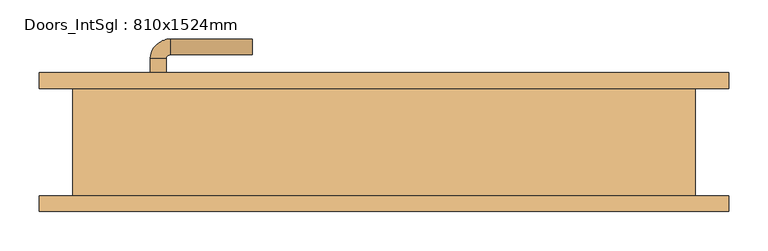
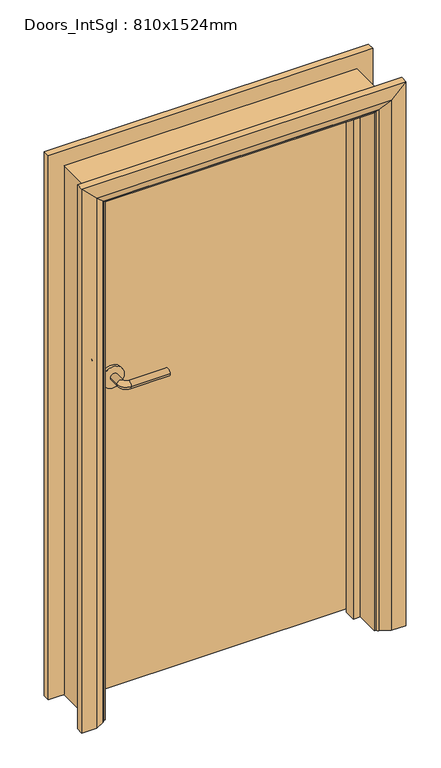
"""IFC4 building model written with IfcOpenShell, lengths in millimetres: door geometry, Doors_IntSgl : 810x1524mm."""

from ifc_helpers import new_model, si_unit, point, frame, frame_2d, origin, place, context, project, spatial, polyline, circle_curve, ellipse_curve, trimmed, segment, composite_curve, outline, extrude, faceted_brep, source, transform, mapped, element, save
from ifc_brep_helpers import plane_surface, cylinder_surface, revolved_surface, advanced_brep


def doors_intsgl_810x1524mm_3577b09a(model_context):
    return source(origin(), model_context, "Body", "SolidModel", [
        advanced_brep(
        [(-298.0, 22.58, 900.0), (-278.0, 22.58, 900.0), (-278.0, -7.42, 900.0), (-298.0, -7.42, 900.0), (-273.0, -12.42, 900.0), (-273.0, -32.42, 900.0), (-168.0, -32.42, 900.0), (-168.0, -12.42, 900.0)],
        [
            (0, 1, circle_curve(frame((-288.0, 22.58, 900.0), z_axis=(0.0, 1.0, 0.0), x_axis=(1.0, 0.0, 0.0)), 10.0)),
            (1, 0, circle_curve(frame((-288.0, 22.58, 900.0), z_axis=(0.0, 1.0, 0.0), x_axis=(1.0, 0.0, 0.0)), 10.0)),
            (1, 2),
            (2, 3, circle_curve(frame((-288.0, -7.42, 900.0), z_axis=(0.0, 1.0, 0.0), x_axis=(1.0, 0.0, 0.0)), 10.0)),
            (3, 0),
            (3, 2, circle_curve(frame((-288.0, -7.42, 900.0), z_axis=(0.0, 1.0, 0.0), x_axis=(1.0, 0.0, 0.0)), 10.0)),
            (4, 5, circle_curve(frame((-273.0, -22.42, 900.0), z_axis=(-1.0, 0.0, 0.0), x_axis=(0.0, 1.0, 0.0)), 10.0)),
            (5, 3, circle_curve(frame((-273.0, -7.42, 900.0), z_axis=(0.0, 0.0, -1.0), x_axis=(-1.0, 0.0, 0.0)), 25.0)),
            (2, 4, circle_curve(frame((-273.0, -7.42, 900.0), z_axis=(0.0, 0.0, 1.0), x_axis=(-1.0, 0.0, 0.0)), 5.0)),
            (5, 4, circle_curve(frame((-273.0, -22.42, 900.0), z_axis=(-1.0, 0.0, 0.0), x_axis=(0.0, 1.0, 0.0)), 10.0)),
            (6, 7, circle_curve(frame((-168.0, -22.42, 900.0), z_axis=(1.0, 0.0, 0.0), x_axis=(0.0, 1.0, 0.0)), 10.0)),
            (7, 6, circle_curve(frame((-168.0, -22.42, 900.0), z_axis=(1.0, 0.0, 0.0), x_axis=(0.0, 1.0, 0.0)), 10.0)),
            (4, 7),
            (6, 5),
        ],
        [
            plane_surface(frame((-288.0, 22.58, 900.0), z_axis=(0.0, 1.0, 0.0), x_axis=(0.0, 0.0, 1.0))),
            cylinder_surface(frame((-288.0, 22.58, 900.0), z_axis=(0.0, 1.0, 0.0), x_axis=(1.0, 0.0, 0.0)), 10.0),
            revolved_surface(trimmed(ellipse_curve(frame((-288.0, -7.42, 900.0), z_axis=(0.0, -1.0, 0.0), x_axis=(1.0, 0.0, 0.0)), 10.0, 10.0), [point((-298.0, -7.42, 900.0))], [point((-278.0, -7.42, 900.0))], True, "CARTESIAN"), (-273.0, -7.42, 900.0), (0.0, 0.0, -1.0)),
            revolved_surface(trimmed(ellipse_curve(frame((-288.0, -7.42, 900.0), z_axis=(0.0, -1.0, 0.0), x_axis=(1.0, 0.0, 0.0)), 10.0, 10.0), [point((-278.0, -7.42, 900.0))], [point((-298.0, -7.42, 900.0))], True, "CARTESIAN"), (-273.0, -7.42, 900.0), (0.0, 0.0, -1.0)),
            plane_surface(frame((-168.0, -22.42, 900.0), z_axis=(1.0, 0.0, 0.0), x_axis=(0.0, 0.0, 1.0))),
            cylinder_surface(frame((-273.0, -22.42, 900.0), z_axis=(-1.0, 0.0, 0.0), x_axis=(0.0, 1.0, 0.0)), 10.0),
        ],
        [
            (0, [[1, 2]]),
            (1, [[3, 4, 5, -2]]),
            (1, [[-5, 6, -3, -1]]),
            (2, [[7, 8, -4, 9]]),
            (3, [[10, -9, -6, -8]]),
            (4, [[11, 12]]),
            (5, [[13, -11, 14, -7]]),
            (5, [[-14, -12, -13, -10]]),
        ],
    ),
        extrude(outline(composite_curve([segment(trimmed(circle_curve(frame_2d((900.0, -290.5)), 30.0), [point((900.0, -320.5))], [point((900.0, -260.5))], False, "CARTESIAN"), True, "CONTINUOUS"), segment(trimmed(circle_curve(frame_2d((900.0, -290.5)), 30.0), [point((900.0, -260.5))], [point((900.0, -320.5))], False, "CARTESIAN"), True, "CONTINUOUS")], self_intersect=False)), frame((0.0, 22.58, 0.0), z_axis=(0.0, 1.0, 0.0), x_axis=(0.0, 0.0, 1.0)), (0.0, 0.0, 1.0), 8.0),
        advanced_brep(
        [(-298.0, 76.58, 900.0), (-278.0, 76.58, 900.0), (-298.0, 106.58, 900.0), (-278.0, 106.58, 900.0), (-273.0, 111.58, 900.0), (-273.0, 131.58, 900.0), (-168.0, 131.58, 900.0), (-168.0, 111.58, 900.0)],
        [
            (0, 1, circle_curve(frame((-288.0, 76.58, 900.0), z_axis=(0.0, -1.0, 0.0), x_axis=(1.0, 0.0, 0.0)), 10.0)),
            (1, 0, circle_curve(frame((-288.0, 76.58, 900.0), z_axis=(0.0, -1.0, 0.0), x_axis=(1.0, 0.0, 0.0)), 10.0)),
            (0, 2),
            (2, 3, circle_curve(frame((-288.0, 106.58, 900.0), z_axis=(0.0, -1.0, 0.0), x_axis=(1.0, 0.0, 0.0)), 10.0)),
            (3, 1),
            (3, 2, circle_curve(frame((-288.0, 106.58, 900.0), z_axis=(0.0, -1.0, 0.0), x_axis=(1.0, 0.0, 0.0)), 10.0)),
            (4, 3, circle_curve(frame((-273.0, 106.58, 900.0), z_axis=(0.0, 0.0, 1.0), x_axis=(-1.0, 0.0, 0.0)), 5.0)),
            (2, 5, circle_curve(frame((-273.0, 106.58, 900.0), z_axis=(0.0, 0.0, -1.0), x_axis=(-1.0, 0.0, 0.0)), 25.0)),
            (5, 4, circle_curve(frame((-273.0, 121.58, 900.0), z_axis=(-1.0, 0.0, 0.0), x_axis=(0.0, -1.0, 0.0)), 10.0)),
            (4, 5, circle_curve(frame((-273.0, 121.58, 900.0), z_axis=(-1.0, 0.0, 0.0), x_axis=(0.0, -1.0, 0.0)), 10.0)),
            (6, 7, circle_curve(frame((-168.0, 121.58, 900.0), z_axis=(1.0, 0.0, 0.0), x_axis=(0.0, -1.0, 0.0)), 10.0)),
            (7, 6, circle_curve(frame((-168.0, 121.58, 900.0), z_axis=(1.0, 0.0, 0.0), x_axis=(0.0, -1.0, 0.0)), 10.0)),
            (5, 6),
            (7, 4),
        ],
        [
            plane_surface(frame((-288.0, 76.58, 900.0), z_axis=(0.0, -1.0, 0.0), x_axis=(0.0, 0.0, 1.0))),
            cylinder_surface(frame((-288.0, 76.58, 900.0), z_axis=(0.0, -1.0, 0.0), x_axis=(1.0, 0.0, 0.0)), 10.0),
            revolved_surface(trimmed(ellipse_curve(frame((-288.0, 106.58, 900.0), z_axis=(0.0, -1.0, 0.0), x_axis=(1.0, 0.0, 0.0)), 10.0, 10.0), [point((-298.0, 106.58, 900.0))], [point((-278.0, 106.58, 900.0))], True, "CARTESIAN"), (-273.0, 106.58, 900.0), (0.0, 0.0, -1.0)),
            revolved_surface(trimmed(ellipse_curve(frame((-288.0, 106.58, 900.0), z_axis=(0.0, -1.0, 0.0), x_axis=(1.0, 0.0, 0.0)), 10.0, 10.0), [point((-278.0, 106.58, 900.0))], [point((-298.0, 106.58, 900.0))], True, "CARTESIAN"), (-273.0, 106.58, 900.0), (0.0, 0.0, -1.0)),
            plane_surface(frame((-168.0, 121.58, 900.0), z_axis=(1.0, 0.0, 0.0), x_axis=(0.0, 0.0, 1.0))),
            cylinder_surface(frame((-273.0, 121.58, 900.0), z_axis=(-1.0, 0.0, 0.0), x_axis=(0.0, -1.0, 0.0)), 10.0),
        ],
        [
            (0, [[1, 2]]),
            (1, [[-1, 3, 4, 5]]),
            (1, [[-2, -5, 6, -3]]),
            (2, [[7, -4, 8, 9]]),
            (3, [[-8, -6, -7, 10]]),
            (4, [[11, 12]]),
            (5, [[-9, 13, -12, 14]]),
            (5, [[-10, -14, -11, -13]]),
        ],
    ),
        extrude(outline(composite_curve([segment(trimmed(circle_curve(frame_2d((900.0, -290.5)), 30.0), [point((900.0, -320.5))], [point((900.0, -260.5))], False, "CARTESIAN"), True, "CONTINUOUS"), segment(trimmed(circle_curve(frame_2d((900.0, -290.5)), 30.0), [point((900.0, -260.5))], [point((900.0, -320.5))], False, "CARTESIAN"), True, "CONTINUOUS")], self_intersect=False)), frame((0.0, 68.58, 0.0), z_axis=(0.0, 1.0, 0.0), x_axis=(0.0, 0.0, 1.0)), (0.0, 0.0, 1.0), 8.0),
        extrude(outline(polyline([(363.0, 30.58), (-363.0, 30.58), (-363.0, 68.58), (363.0, 68.58), (363.0, 30.58)])), frame((0.0, 0.0, 8.0), z_axis=(0.0, 0.0, 1.0), x_axis=(1.0, 0.0, 0.0)), (0.0, 0.0, 1.0), 1474.0),
        advanced_brep(
        [(440.0, 88.58, 0.0), (440.0, 68.58, 0.0), (370.0, 68.58, 0.0), (374.0, 74.58, 0.0), (400.0, 88.58, 0.0), (440.0, 88.58, 1559.0), (440.0, 68.58, 1559.0), (-440.0, 68.58, 1559.0), (-440.0, 68.58, 0.0), (-370.0, 68.58, 0.0), (-370.0, 68.58, 1489.0), (370.0, 68.58, 1489.0), (374.0, 74.58, 1493.0), (400.0, 88.58, 1519.0), (-400.0, 88.58, 1519.0), (-400.0, 88.58, 0.0), (-440.0, 88.58, 0.0), (-440.0, 88.58, 1559.0), (-374.0, 74.58, 1493.0), (-374.0, 74.58, 0.0)],
        [
            (0, 1),
            (1, 2),
            (2, 3, circle_curve(frame((378.0, 67.58, 0.0), z_axis=(0.0, 0.0, -1.0), x_axis=(1.0, 0.0, 0.0)), 8.0622577)),
            (3, 4),
            (4, 0),
            (0, 5),
            (5, 6),
            (6, 1),
            (6, 7),
            (7, 8),
            (8, 9),
            (9, 10),
            (10, 11),
            (11, 2),
            (11, 12, ellipse_curve(frame((378.0, 67.58, 1497.0), z_axis=(0.7071067811865475, 0.0, -0.7071067811865475), x_axis=(-0.7071067811865474, 0.0, -0.7071067811865476)), 11.4017543, 8.0622577)),
            (12, 3),
            (12, 13),
            (13, 4),
            (13, 14),
            (14, 15),
            (15, 16),
            (16, 17),
            (17, 5),
            (17, 7),
            (10, 18, ellipse_curve(frame((-378.0, 67.58, 1497.0), z_axis=(0.7071067811865475, 0.0, 0.7071067811865475), x_axis=(0.7071067811865476, 0.0, -0.7071067811865474)), 11.4017543, 8.0622577)),
            (18, 12),
            (18, 14),
            (15, 19),
            (19, 9, circle_curve(frame((-378.0, 67.58, 0.0), z_axis=(0.0, 0.0, -1.0), x_axis=(-1.0, 0.0, 0.0)), 8.0622577)),
            (8, 16),
            (19, 18),
        ],
        [
            plane_surface(frame((370.0, 68.58, 0.0), z_axis=(0.0, 0.0, -1.0), x_axis=(0.0, -1.0, 0.0))),
            plane_surface(frame((440.0, 88.58, 0.0), z_axis=(1.0, 0.0, 0.0), x_axis=(0.0, 0.0, 1.0))),
            plane_surface(frame((440.0, 68.58, 0.0), z_axis=(0.0, -1.0, 0.0), x_axis=(0.0, 0.0, 1.0))),
            cylinder_surface(frame((378.0, 67.58, 0.0), z_axis=(0.0, 0.0, -1.0), x_axis=(1.0, 0.0, 0.0)), 8.0622577),
            plane_surface(frame((374.0, 74.58, 0.0), z_axis=(-0.4740998230350126, 0.880471099922178, 0.0), x_axis=(0.0, 0.0, 1.0))),
            plane_surface(frame((400.0, 88.58, 0.0), z_axis=(0.0, 1.0, 0.0), x_axis=(0.0, 0.0, 1.0))),
            plane_surface(frame((440.0, 88.58, 1559.0), z_axis=(0.0, 0.0, 1.0), x_axis=(-1.0, 0.0, 0.0))),
            cylinder_surface(frame((370.0, 67.58, 1497.0), z_axis=(1.0, 0.0, 0.0), x_axis=(0.0, 0.0, 1.0)), 8.0622577),
            plane_surface(frame((374.0, 74.58, 1493.0), z_axis=(0.0, 0.8804710999221764, -0.4740998230350154), x_axis=(-1.0, 0.0, 0.0))),
            plane_surface(frame((-370.0, 68.58, 0.0), z_axis=(0.0, 0.0, -1.0), x_axis=(0.0, -1.0, 0.0))),
            plane_surface(frame((-440.0, 88.58, 1559.0), z_axis=(-1.0, 0.0, 0.0), x_axis=(0.0, 0.0, -1.0))),
            cylinder_surface(frame((-378.0, 67.58, 1489.0), z_axis=(0.0, 0.0, 1.0), x_axis=(-1.0, 0.0, 0.0)), 8.0622577),
            plane_surface(frame((-374.0, 74.58, 1493.0), z_axis=(0.47409982303501824, 0.8804710999221749, 0.0), x_axis=(0.0, 0.0, -1.0))),
        ],
        [
            (0, [[1, 2, 3, 4, 5]]),
            (1, [[-1, 6, 7, 8]]),
            (2, [[-2, -8, 9, 10, 11, 12, 13, 14]]),
            (3, [[-3, -14, 15, 16]]),
            (4, [[-4, -16, 17, 18]]),
            (5, [[-5, -18, 19, 20, 21, 22, 23, -6]]),
            (6, [[-7, -23, 24, -9]]),
            (7, [[-15, -13, 25, 26]]),
            (8, [[-17, -26, 27, -19]]),
            (9, [[-21, 28, 29, -11, 30]]),
            (10, [[-24, -22, -30, -10]]),
            (11, [[-25, -12, -29, 31]]),
            (12, [[-27, -31, -28, -20]]),
        ],
    ),
        advanced_brep(
        [(-440.0, -88.58, 0.0), (-440.0, -68.58, 0.0), (-370.0, -68.58, 0.0), (-374.0, -74.58, 0.0), (-400.0, -88.58, 0.0), (-440.0, -88.58, 1559.0), (-440.0, -68.58, 1559.0), (-370.0, -68.58, 1489.0), (-374.0, -74.58, 1493.0), (-400.0, -88.58, 1519.0), (440.0, -88.58, 1559.0), (440.0, -68.58, 1559.0), (370.0, -68.58, 1489.0), (374.0, -74.58, 1493.0), (400.0, -88.58, 1519.0), (440.0, -88.58, 0.0), (400.0, -88.58, 0.0), (374.0, -74.58, 0.0), (370.0, -68.58, 0.0), (440.0, -68.58, 0.0)],
        [
            (0, 1),
            (1, 2),
            (2, 3, circle_curve(frame((-378.0, -67.58, 0.0), z_axis=(0.0, 0.0, -1.0), x_axis=(-1.0, 0.0, 0.0)), 8.0622577)),
            (3, 4),
            (4, 0),
            (0, 5),
            (5, 6),
            (6, 1),
            (6, 7),
            (7, 2),
            (7, 8, ellipse_curve(frame((-378.0, -67.58, 1497.0), z_axis=(-0.7071067811865475, 0.0, -0.7071067811865475), x_axis=(0.7071067811865474, 0.0, -0.7071067811865476)), 11.4017543, 8.0622577)),
            (8, 3),
            (8, 9),
            (9, 4),
            (9, 5),
            (5, 10),
            (10, 11),
            (11, 6),
            (11, 12),
            (12, 7),
            (12, 13, ellipse_curve(frame((378.0, -67.58, 1497.0), z_axis=(-0.7071067811865475, 0.0, 0.7071067811865475), x_axis=(-0.7071067811865476, 0.0, -0.7071067811865474)), 11.4017543, 8.0622577)),
            (13, 8),
            (13, 14),
            (14, 9),
            (14, 10),
            (15, 16),
            (16, 17),
            (17, 18, circle_curve(frame((378.0, -67.58, 0.0), z_axis=(0.0, 0.0, -1.0), x_axis=(1.0, 0.0, 0.0)), 8.0622577)),
            (18, 19),
            (19, 15),
            (10, 15),
            (19, 11),
            (18, 12),
            (17, 13),
            (16, 14),
        ],
        [
            plane_surface(frame((-370.0, -141.3810989, 0.0), z_axis=(0.0, 0.0, -1.0), x_axis=(1.0, 0.0, 0.0))),
            plane_surface(frame((-440.0, -88.58, 0.0), z_axis=(-1.0, 0.0, 0.0), x_axis=(0.0, 0.0, 1.0))),
            plane_surface(frame((-440.0, -68.58, 0.0), z_axis=(0.0, 1.0, 0.0), x_axis=(0.0, 0.0, 1.0))),
            cylinder_surface(frame((-378.0, -67.58, 0.0), z_axis=(0.0, 0.0, -1.0), x_axis=(-1.0, 0.0, 0.0)), 8.0622577),
            plane_surface(frame((-374.0, -74.58, 0.0), z_axis=(0.4740998230350183, -0.8804710999221749, 0.0), x_axis=(0.0, 0.0, 1.0))),
            plane_surface(frame((-400.0, -88.58, 0.0), z_axis=(0.0, -1.0, 0.0), x_axis=(0.0, 0.0, 1.0))),
            plane_surface(frame((-440.0, -88.58, 1559.0), z_axis=(0.0, 0.0, 1.0), x_axis=(1.0, 0.0, 0.0))),
            plane_surface(frame((-440.0, -68.58, 1559.0), z_axis=(0.0, 1.0, 0.0), x_axis=(1.0, 0.0, 0.0))),
            cylinder_surface(frame((-370.0, -67.58, 1497.0), z_axis=(-1.0, 0.0, 0.0), x_axis=(0.0, 0.0, 1.0)), 8.0622577),
            plane_surface(frame((-374.0, -74.58, 1493.0), z_axis=(0.0, -0.8804710999221749, -0.4740998230350183), x_axis=(1.0, 0.0, 0.0))),
            plane_surface(frame((-400.0, -88.58, 1519.0), z_axis=(0.0, -1.0, 0.0), x_axis=(1.0, 0.0, 0.0))),
            plane_surface(frame((370.0, -141.3810989, 0.0), z_axis=(0.0, 0.0, -1.0), x_axis=(-1.0, 0.0, 0.0))),
            plane_surface(frame((440.0, -88.58, 1559.0), z_axis=(1.0, 0.0, 0.0), x_axis=(0.0, 0.0, -1.0))),
            plane_surface(frame((440.0, -68.58, 1559.0), z_axis=(0.0, 1.0, 0.0), x_axis=(0.0, 0.0, -1.0))),
            cylinder_surface(frame((378.0, -67.58, 1489.0), z_axis=(0.0, 0.0, 1.0), x_axis=(1.0, 0.0, 0.0)), 8.0622577),
            plane_surface(frame((374.0, -74.58, 1493.0), z_axis=(-0.4740998230350183, -0.8804710999221749, 0.0), x_axis=(0.0, 0.0, -1.0))),
            plane_surface(frame((400.0, -88.58, 1519.0), z_axis=(0.0, -1.0, 0.0), x_axis=(0.0, 0.0, -1.0))),
        ],
        [
            (0, [[1, 2, 3, 4, 5]]),
            (1, [[-1, 6, 7, 8]]),
            (2, [[-2, -8, 9, 10]]),
            (3, [[-3, -10, 11, 12]]),
            (4, [[-4, -12, 13, 14]]),
            (5, [[-5, -14, 15, -6]]),
            (6, [[-7, 16, 17, 18]]),
            (7, [[-9, -18, 19, 20]]),
            (8, [[-11, -20, 21, 22]]),
            (9, [[-13, -22, 23, 24]]),
            (10, [[-15, -24, 25, -16]]),
            (11, [[26, 27, 28, 29, 30]]),
            (12, [[-17, 31, -30, 32]]),
            (13, [[-19, -32, -29, 33]]),
            (14, [[-21, -33, -28, 34]]),
            (15, [[-23, -34, -27, 35]]),
            (16, [[-25, -35, -26, -31]]),
        ],
    ),
        faceted_brep([(-365.0, 68.58, 0.0), (-365.0, -68.58, 0.0), (-397.0, -68.58, 0.0), (-397.0, 68.58, 0.0), (-365.0, 68.58, 1484.0), (-365.0, -68.58, 1484.0), (-397.0, -68.58, 1516.0), (-397.0, 68.58, 1516.0), (365.0, 68.58, 1484.0), (365.0, -68.58, 1484.0), (397.0, -68.58, 1516.0), (397.0, 68.58, 1516.0), (365.0, 68.58, 0.0), (397.0, 68.58, 0.0), (397.0, -68.58, 0.0), (365.0, -68.58, 0.0)], [[[0, 1, 2, 3]], [[1, 0, 4, 5]], [[2, 1, 5, 6]], [[3, 2, 6, 7]], [[0, 3, 7, 4]], [[5, 4, 8, 9]], [[6, 5, 9, 10]], [[7, 6, 10, 11]], [[4, 7, 11, 8]], [[12, 13, 14, 15]], [[9, 8, 12, 15]], [[10, 9, 15, 14]], [[11, 10, 14, 13]], [[8, 11, 13, 12]]]),
        extrude(outline(polyline([(0.0, -365.0), (0.0, -346.0), (1465.0, -346.0), (1465.0, 346.0), (0.0, 346.0), (0.0, 365.0), (1484.0, 365.0), (1484.0, -365.0), (0.0, -365.0)])), frame((0.0, -3.42, 0.0), z_axis=(0.0, 1.0, 0.0), x_axis=(0.0, 0.0, 1.0)), (0.0, 0.0, 1.0), 32.0),
    ])


if __name__ == "__main__":
    model = new_model("IFC4")
    model_context = context("Model", 3, world=origin())
    ifc_project = project(units=[si_unit("LENGTHUNIT", "METRE", prefix="MILLI")], contexts=[model_context])
    site = spatial("IfcSite", under=ifc_project)
    building = spatial("IfcBuilding", under=site)
    placement = place(None, origin())
    doors_intsgl_810x1524mm_shape = doors_intsgl_810x1524mm_3577b09a(model_context)
    element("IfcDoor", 1, ObjectType="Doors_IntSgl : 810x1524mm", at=placement, inside=building, context=model_context, shape_type="MappedRepresentation", body=[
        mapped(doors_intsgl_810x1524mm_shape, transform((0.0, 0.0, 0.0), x_axis=(1.0, 0.0, 0.0), y_axis=(0.0, 1.0, 0.0), z_axis=(0.0, 0.0, 1.0))),
    ])
    save(model, "model.ifc")

# Revit data of these elements
# Type "Doors_IntSgl : 810x1524mm"
#   Construction Type Id = "MDOOR"
#   Type Mark = "42"
#   Type Comments = "Internal Single"
#   Operation = "SingleSwingRight"
#   Manufacturer = "Revit"
#   Keynote = "L20"
#   Description = "Internal Single Door"
#   Analytic Construction = "Metal"
#   UnderCut = 8 mm
#   Tolerance = 2 mm
#   Thickness = 38 mm
#   Thermal Resistance (R) = 0.270117 (m²·K)/W
#   Structural Tolerance = 8 mm
#   StopDepth = 32 mm
#   Stop Thickness = 19 mm
#   Rough Width = 810 mm
#   Rough Height = 1524 mm
#   Height to Top Lock Rail = 1000 mm
#   Heat Transfer Coefficient (U) = 3.7021 W/(m²·K)
#   Handle Z Distance = 900 mm
#   Handle X Distance = 75 mm
#   Frame Thickness = 32 mm
#   Door Panel Width = 726 mm
#   Door Panel Thickness = 38 mm
#   Door Panel Offset = 0 mm
#   Height = 1524 mm
#   Width = 810 mm
#   Door Panel Height = 1474 mm
#   Architrave Setback = 5 mm
#   Define Thermal Properties by = 1
#   Vis - Ironmongery = yes
#   Material Ironmongery = Door - Handle
#   Material Frame = Door - Frame/Mullion (1)
#   Material Door = Door - Panel
#   Material Architrave = Door - Architrave
#   Visual Light Transmittance = 0
#   Solar Heat Gain Coefficient = 0
#   Function = (empty or 0)
#   Wall Closure = (empty or 0)
# Element 1 (IfcDoor, "Doors_IntSgl : 810x1524mm")
#   Materials on its faces: "Door - Architrave", "Door - Handle", "Door - Frame/Mullion (1)", "Door - Panel"
# Materials
#   "Door - Handle": colour RGB 0 0 0, transparency 0, Keynote = "P21", Cost = 0
#   "Door - Frame/Mullion (1)": class "Wood", colour RGB 212 179 113, transparency 0, Keynote = "L20", Cost = 0
#   "Door - Panel": class "Wood", colour RGB 210 159 95, transparency 0, Keynote = "L20", Cost = 0
#   "Door - Architrave": class "Wood", colour RGB 154 90 5, transparency 0, Keynote = "P20", Cost = 0
